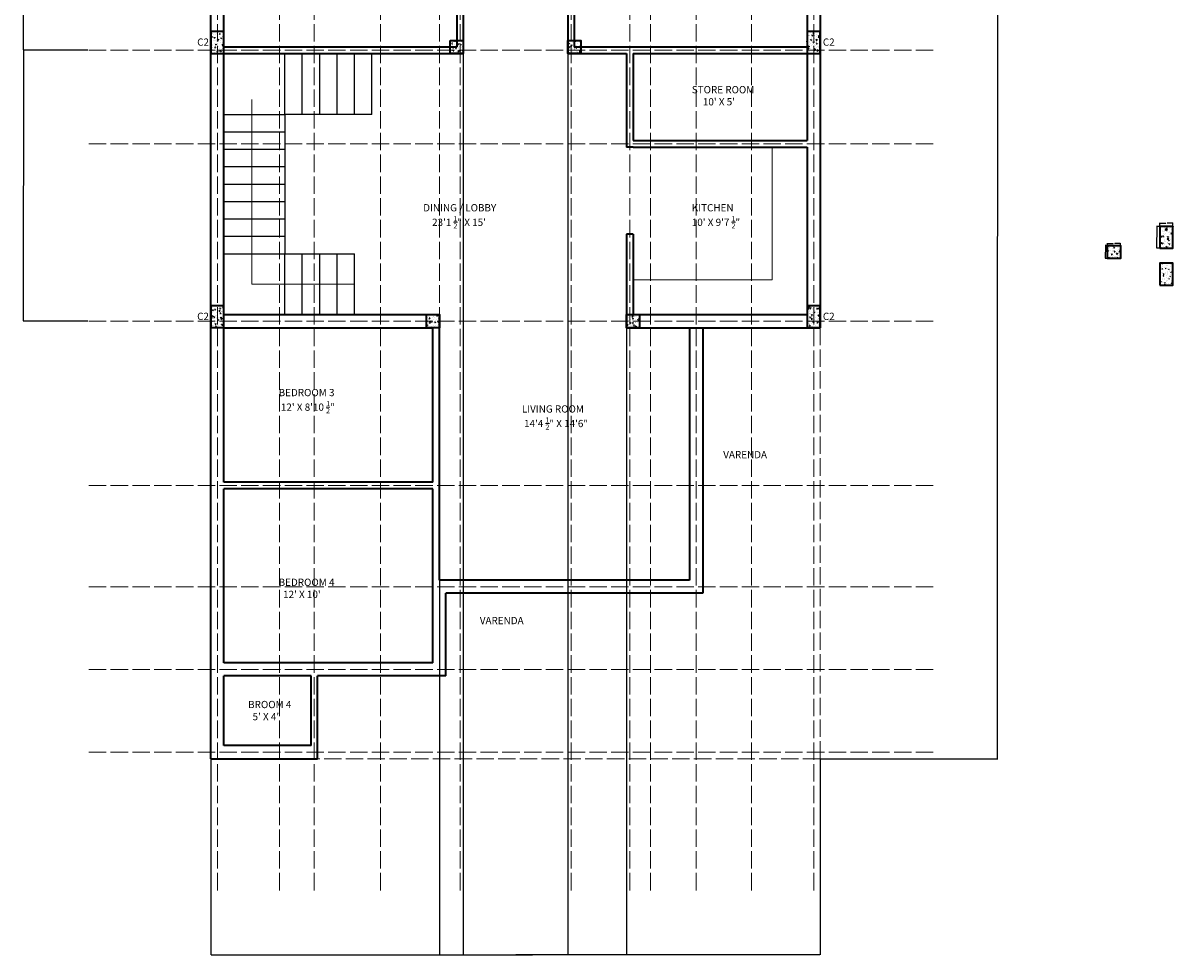
# Model space of a CAD drawing. Units: inches. Extents: x 1159 to 4240, y 1112 to 2085.
# Tile 11 of 13: x 2561 to 3354, y 1112 to 1755. Entities that reach past the tile are written whole.
import ezdxf

# ---------------------------------------------------------------- set-up
doc = ezdxf.new("R2010")
doc.units = ezdxf.units.IN
doc.linetypes.add('ACAD_ISO02W100', pattern=[15, 12, -3])
for name, color, linetype, lineweight in [('A-ANNO-DIMS', 2, 'Continuous', 18), ('A-ANNO-SYMB', 150, 'Continuous', 18), ('A-AREA-IDEN', 30, 'Continuous', 18), ('A-COLS-PATT', 120, 'Continuous', 13), ('A-FLOR-EDGE', 1, 'ACAD_ISO02W100', 18), ('A-GRID', 8, 'ACAD_ISO02W100', 13), ('COLUMN', 120, 'Continuous', 35), ('column no', 210, 'Continuous', 18), ('KITCHEN', 1, 'Continuous', 18), ('STAIRCASE', 150, 'Continuous', 25), ('WALL', 7, 'Continuous', 35)]:
    doc.layers.add(name, color=color, linetype=linetype, lineweight=lineweight)
doc.styles.get("Standard").update_dxf_attribs({"font": 'arial.ttf'})
doc.dimstyles.get("Standard").update_dxf_attribs({"dimtxt": 0.18, "dimasz": 0.18, "dimexe": 0.18, "dimexo": 0.0625, "dimgap": 0.09, "dimtad": 0, "dimtih": 1, "dimtoh": 1, "dimdec": 4, "dimzin": 0, "dimdsep": 46, "dimtxsty": 'Standard', "dimcen": 0.09, "dimadec": 0, "dimazin": 0, "dimtfac": 1, "dimtdec": 4, "dimtofl": 0, "dimtmove": 0, "dimatfit": 3, "dimfxl": 1, "dimtolj": 1, "dimtzin": 0, "dimarcsym": 0})

# ---------------------------------------------------------------- blocks, each defined once
blk = doc.blocks.new('column')
at = {"layer": 'COLUMN'}
h = blk.add_hatch(dxfattribs=at)
h.set_pattern_fill('AR-CONC', color=256, scale=0.025)
h.set_pattern_definition([(50, (-3308.5408, -1592.3894), (4.5546167, -0.398477), [0.47625, -5.23875]), (355, (-3308.541, -1592.3894), (-0.8810855, 4.776421), [0.381, -4.1910146]), (100.45144, (-3308.1612, -1592.4226), (3.673531, 4.377944), [0.40475, -4.452256]), (46.1842, (-3308.541, -1591.1194), (6.776976, -1.051058), [0.714375, -7.858125]), (96.63556, (-3307.976, -1591.207), (5.935103, 6.185653), [0.607126, -6.67839]), (351.18415, (-3308.541, -1591.1194), (5.935103, 6.185653), [0.571499, -6.286493]), (21, (-3307.9058, -1591.437), (3.7903598, -2.55663), [0.47625, -5.23875]), (326, (-3307.906, -1591.437), (1.545051, 4.604699), [0.381, -4.191]), (71.45144, (-3307.59, -1591.65), (5.3354105, 2.048069), [0.40475, -4.4522484]), (37.5, (-3308.5408, -1592.3894), (0.0772151, 2.113876), [0, -4.1402, 0, -4.2545, 0, -4.206875]), (7.5, (-3308.5408, -1592.3894), (1.6704916, 2.5045144), [0, -2.4257, 0, -4.04495, 0, -1.603375]), (327.5, (-3309.9568, -1592.3894), (3.3897649, -0.1432186), [0, -1.5875, 0, -4.953, 0, -6.57225]), (317.5, (-3310.5918, -1592.3894), (3.7032295, 0.6356623), [0, -2.06375, 0, -3.2893, 0, -4.66725])])
h.paths.add_polyline_path([(0, 9), (0, 0), (9, 0), (9, 9)])
blk.add_lwpolyline([(0, 9), (9, 9), (9, 0), (0, 0)], close=True, dxfattribs=at)
blk = doc.blocks.new('colum 1')
at = {"layer": 'COLUMN'}
h = blk.add_hatch(dxfattribs=at)
h.set_pattern_fill('AR-CONC', color=256, scale=0.025)
h.set_pattern_definition([(50, (-3344.692, -1599.4877), (4.5546167, -0.398477), [0.47625, -5.23875]), (355, (-3344.692, -1599.4877), (-0.8810855, 4.776421), [0.381, -4.1910146]), (100.45144, (-3344.3125, -1599.521), (3.673531, 4.377944), [0.40475, -4.452256]), (46.1842, (-3344.692, -1598.218), (6.776976, -1.051058), [0.714375, -7.858125]), (96.63556, (-3344.127, -1598.305), (5.935103, 6.185653), [0.607126, -6.67839]), (351.18415, (-3344.692, -1598.218), (5.935103, 6.185653), [0.571499, -6.286493]), (21, (-3344.057, -1598.5352), (3.7903598, -2.55663), [0.47625, -5.23875]), (326, (-3344.057, -1598.5352), (1.545051, 4.604699), [0.381, -4.191]), (71.45144, (-3343.741, -1598.7483), (5.3354105, 2.048069), [0.40475, -4.4522484]), (37.5, (-3344.692, -1599.4877), (0.0772151, 2.113876), [0, -4.1402, 0, -4.2545, 0, -4.206875]), (7.5, (-3344.692, -1599.4877), (1.6704916, 2.5045144), [0, -2.4257, 0, -4.04495, 0, -1.603375]), (327.5, (-3346.1081, -1599.4877), (3.3897649, -0.1432186), [0, -1.5875, 0, -4.953, 0, -6.57225]), (317.5, (-3346.743, -1599.4877), (3.7032295, 0.6356623), [0, -2.06375, 0, -3.2893, 0, -4.66725])])
h.paths.add_polyline_path([(9, 15), (0, 15), (0, 0), (9, 0)])
blk.add_lwpolyline([(0, 0), (9, 0), (9, 15), (0, 15)], close=True, dxfattribs=at)
blk = doc.blocks.new('HOUSE-35x60-WALL-LAYOUT')
for p, q in [((0, 0), (0, 720)), ((0, 720), (420, 720)), ((420, 720), (420, 297)), ((9, 711), (45, 711)), ((9, 634.5), (9, 711)), ((45, 634.5), (45, 711)), ((49.5, 639), (49.5, 711)), ((49.5, 711), (112.5, 711)), ((112.5, 639), (112.5, 711)), ((121.5, 639), (121.5, 711)), ((121.5, 711), (298.5, 711)), ((298.5, 711), (298.5, 639)), ((307.5, 711), (307.5, 639)), ((307.5, 711), (370.5, 711)), ((370.5, 711), (370.5, 639)), ((375, 711), (375, 634.5)), ((375, 711), (411, 711)), ((411, 711), (411, 634.5)), ((9, 490.5), (9, 634.5)), ((45, 634.5), (169.5, 634.5)), ((49.5, 639), (112.5, 639)), ((121.5, 639), (298.5, 639)), ((169.5, 634.5), (169.5, 490.5)), ((174, 634.5), (174, 531)), ((174, 634.5), (246, 634.5)), ((246, 634.5), (246, 531)), ((250.5, 634.5), (250.5, 490.5)), ((250.5, 634.5), (375, 634.5)), ((307.5, 639), (370.5, 639)), ((411, 634.5), (411, 490.5)), ((174, 531), (246, 531)), ((174, 526.5), (246, 526.5)), ((174, 526.5), (174, 486)), ((246, 526.5), (246, 486)), ((9, 490.5), (169.5, 490.5)), ((9, 486), (174, 486)), ((9, 306), (9, 486)), ((246, 486), (286.5, 486)), ((250.5, 490.5), (411, 490.5)), ((286.5, 486), (286.5, 421.5)), ((291, 486), (291, 426)), ((291, 486), (411, 486)), ((411, 486), (411, 426)), ((291, 421.5), (286.5, 421.5)), ((291, 426), (411, 426)), ((291, 421.5), (411, 421.5)), ((411, 421.5), (411, 306)), ((291, 361.5), (286.5, 361.5)), ((286.5, 361.5), (286.5, 297)), ((291, 361.5), (291, 306)), ((9, 306), (157.5, 306)), ((157.5, 190.5), (157.5, 306)), ((291, 306), (411, 306)), ((9, 297), (153, 297)), ((9, 190.5), (9, 297)), ((153, 190.5), (153, 297)), ((286.5, 297), (420, 297)), ((330, 297), (330, 123)), ((339, 297), (339, 114)), ((153, 190.5), (9, 190.5)), ((157.5, 123), (157.5, 190.5)), ((9, 66), (9, 186)), ((153, 186), (9, 186)), ((153, 66), (153, 186)), ((330, 123), (157.5, 123)), ((162, 57), (162, 114)), ((339, 114), (162, 114)), ((153, 66), (9, 66)), ((9, 9), (9, 57)), ((69, 57), (9, 57)), ((69, 9), (69, 57)), ((162, 57), (73.5, 57)), ((73.5, 0), (73.5, 57)), ((69, 9), (9, 9)), ((0, 0), (73.5, 0))]:
    blk.add_line(p, q)
blk = doc.blocks.new('STAIR-THREE-FLIGHT')
for p, q in [((42, 138), (42, 180)), ((54, 138), (54, 180)), ((66, 138), (66, 180)), ((78, 138), (78, 180)), ((90, 138), (90, 180)), ((102, 138), (102, 180)), ((0, 138), (42, 138)), ((102, 138), (42, 138)), ((42, 138), (42, 42)), ((0, 126), (42, 126)), ((0, 114), (42, 114)), ((0, 102), (42, 102)), ((0, 90), (42, 90)), ((0, 78), (42, 78)), ((0, 66), (42, 66)), ((0, 54), (42, 54)), ((0, 42), (42, 42)), ((42, 0), (42, 42)), ((42, 42), (90, 42)), ((54, 0), (54, 42)), ((66, 0), (66, 42)), ((78, 0), (78, 42)), ((90, 0), (90, 42))]:
    blk.add_line(p, q)
blk = doc.blocks.new('STAIR-PATH-ARROW')
blk.add_lwpolyline([(0, 127.38, 0, 0, 0), (0, 143.35, 0, 0, 0), (58.69, 143.35, 4, 0, 0), (70.69, 143.35, 0, 0, 0)], format="xyseb")
blk.add_lwpolyline([(70.69, 0), (0, 0), (0, 127.38)])
blk = doc.blocks.new('KITCHEN-COUNTER-L')
for p in [(96, 91.5), (0, 0)]:
    blk.add_line(p, (96, 0))
blk = doc.blocks.new('HOUSE-35x60-SETTING-OUT-GRID')
for p, q in [((89.32, 0), (89.32, 883.25)), ((132.07, 0), (132.07, 883.25)), ((156.07, 0), (156.07, 883.25)), ((201.82, 0), (201.82, 883.25)), ((242.32, 0), (242.32, 883.25)), ((256.57, 0), (256.57, 883.25)), ((333.07, 0), (333.07, 883.25)), ((373.57, 0), (373.57, 883.25)), ((387.82, 0), (387.82, 883.25)), ((419.32, 0), (419.32, 883.25)), ((457.57, 0), (457.57, 883.25)), ((500.32, 0), (500.32, 883.25)), ((582.7, 806.25), (0, 806.25)), ((582.7, 727.5), (0, 727.5)), ((582.7, 619.5), (0, 619.5)), ((582.7, 579), (0, 579)), ((582.7, 514.5), (0, 514.5)), ((582.7, 392.25), (0, 392.25)), ((582.7, 279), (0, 279)), ((582.7, 209.25), (0, 209.25)), ((582.7, 152.25), (0, 152.25)), ((582.7, 95.25), (0, 95.25))]:
    blk.add_line(p, q)
blk = doc.blocks.new('*D12')
at = {"layer": 'A-ANNO-DIMS', "color": 0, "lineweight": -2, "transparency": 16777216}
for p, q in [((3308.54, 1601.45), (3308.54, 1602.92)), ((3308.72, 1602.74), (3312.39, 1602.74)), ((3317.36, 1602.74), (3313.69, 1602.74)), ((3317.54, 1601.45), (3317.54, 1602.92))]:
    blk.add_line(p, q, dxfattribs=at)
at = {"layer": 'A-ANNO-DIMS', "color": 0, "lineweight": 100, "transparency": 16777216}
for points in [[(3308.72, 1602.77), (3308.72, 1602.71), (3308.54, 1602.74)], [(3317.36, 1602.77), (3317.36, 1602.71), (3317.54, 1602.74)]]:
    blk.add_solid(points, dxfattribs=at)
at = {"layer": 'Defpoints', "color": 0, "lineweight": 100, "transparency": 16777216}
for p in [(3308.54, 1601.39), (3317.54, 1602.74), (3317.54, 1601.39)]:
    blk.add_point(p, dxfattribs=at)
at = {"layer": 'A-ANNO-DIMS', "color": 0, "transparency": 16777216, "insert": (3313.04, 1602.74), "char_height": 0.18, "attachment_point": 5}
blk.add_mtext('\\A1;C1 9 TYP.', dxfattribs=at)
blk = doc.blocks.new('*D13')
at = {"layer": 'A-ANNO-DIMS', "color": 0, "lineweight": -2, "transparency": 16777216}
for p, q in [((3308.48, 1601.39), (3307.01, 1601.39)), ((3307.19, 1601.21), (3307.19, 1597.07)), ((3307.19, 1592.57), (3307.19, 1596.71)), ((3308.48, 1592.39), (3307.01, 1592.39))]:
    blk.add_line(p, q, dxfattribs=at)
at = {"layer": 'A-ANNO-DIMS', "color": 0, "lineweight": 100, "transparency": 16777216}
for points in [[(3307.16, 1601.21), (3307.22, 1601.21), (3307.19, 1601.39)], [(3307.16, 1592.57), (3307.22, 1592.57), (3307.19, 1592.39)]]:
    blk.add_solid(points, dxfattribs=at)
at = {"layer": 'Defpoints', "color": 0, "lineweight": 100, "transparency": 16777216}
for p in [(3307.19, 1601.39), (3308.54, 1601.39), (3308.54, 1592.39)]:
    blk.add_point(p, dxfattribs=at)
at = {"layer": 'A-ANNO-DIMS', "color": 0, "transparency": 16777216, "insert": (3307.19, 1596.89), "char_height": 0.18, "attachment_point": 5}
blk.add_mtext('\\A1;9 TYP.', dxfattribs=at)
blk = doc.blocks.new('*D14')
at = {"layer": 'A-ANNO-DIMS', "color": 0, "lineweight": -2, "transparency": 16777216}
for p, q in [((3344.63, 1614.49), (3342.26, 1614.49)), ((3342.44, 1614.31), (3342.44, 1607.17)), ((3342.44, 1599.67), (3342.44, 1606.8)), ((3344.63, 1599.49), (3342.26, 1599.49))]:
    blk.add_line(p, q, dxfattribs=at)
at = {"layer": 'A-ANNO-DIMS', "color": 0, "lineweight": 100, "transparency": 16777216}
for points in [[(3342.41, 1614.31), (3342.47, 1614.31), (3342.44, 1614.49)], [(3342.41, 1599.67), (3342.47, 1599.67), (3342.44, 1599.49)]]:
    blk.add_solid(points, dxfattribs=at)
at = {"layer": 'Defpoints', "color": 0, "lineweight": 100, "transparency": 16777216}
for p in [(3342.44, 1614.49), (3344.69, 1614.49), (3344.69, 1599.49)]:
    blk.add_point(p, dxfattribs=at)
at = {"layer": 'A-ANNO-DIMS', "color": 0, "transparency": 16777216, "insert": (3342.44, 1606.99), "char_height": 0.18, "attachment_point": 5}
blk.add_mtext('\\A1;C2 15 TYP.', dxfattribs=at)
blk = doc.blocks.new('*D15')
at = {"layer": 'A-ANNO-DIMS', "color": 0, "lineweight": -2, "transparency": 16777216}
for p, q in [((3344.69, 1614.55), (3344.69, 1616.92)), ((3344.87, 1616.74), (3348.73, 1616.74)), ((3353.51, 1616.74), (3349.65, 1616.74)), ((3353.69, 1614.55), (3353.69, 1616.92))]:
    blk.add_line(p, q, dxfattribs=at)
at = {"layer": 'A-ANNO-DIMS', "color": 0, "lineweight": 100, "transparency": 16777216}
for points in [[(3344.87, 1616.77), (3344.87, 1616.71), (3344.69, 1616.74)], [(3353.51, 1616.77), (3353.51, 1616.71), (3353.69, 1616.74)]]:
    blk.add_solid(points, dxfattribs=at)
at = {"layer": 'Defpoints', "color": 0, "lineweight": 100, "transparency": 16777216}
for p in [(3344.69, 1614.49), (3353.69, 1616.74), (3353.69, 1614.49)]:
    blk.add_point(p, dxfattribs=at)
at = {"layer": 'A-ANNO-DIMS', "color": 0, "transparency": 16777216, "insert": (3349.19, 1616.74), "char_height": 0.18, "attachment_point": 5}
blk.add_mtext('\\A1;9 TYP.', dxfattribs=at)
blk = doc.blocks.new('*D24')
at = {"layer": 'A-ANNO-DIMS', "color": 0, "lineweight": -2, "transparency": 16777216}
for p, q in [((2690.48, 1247.64), (2690.48, 1112.42)), ((3110.48, 1247.64), (3110.48, 1112.42)), ((2690.66, 1112.6), (2900.19, 1112.6)), ((3110.3, 1112.6), (2900.78, 1112.6))]:
    blk.add_line(p, q, dxfattribs=at)
at = {"layer": 'A-ANNO-DIMS', "color": 0, "lineweight": 100, "transparency": 16777216}
for points in [[(2690.66, 1112.63), (2690.66, 1112.57), (2690.48, 1112.6)], [(3110.3, 1112.63), (3110.3, 1112.57), (3110.48, 1112.6)]]:
    blk.add_solid(points, dxfattribs=at)
at = {"layer": 'Defpoints', "color": 0, "lineweight": 100, "transparency": 16777216}
for p in [(2690.48, 1247.7), (3110.48, 1247.7), (3110.48, 1112.6)]:
    blk.add_point(p, dxfattribs=at)
at = {"layer": 'A-ANNO-DIMS', "color": 0, "transparency": 16777216, "insert": (2900.48, 1112.6), "char_height": 0.18, "attachment_point": 5}
blk.add_mtext('\\A1;420', dxfattribs=at)
blk = doc.blocks.new('*D25')
at = {"layer": 'A-ANNO-DIMS', "color": 0, "lineweight": -2, "transparency": 16777216}
for p, q in [((3110.55, 1967.7), (3232.9, 1967.7)), ((3232.72, 1967.52), (3232.72, 1607.88)), ((3232.72, 1247.88), (3232.72, 1607.52)), ((3110.55, 1247.7), (3232.9, 1247.7))]:
    blk.add_line(p, q, dxfattribs=at)
at = {"layer": 'A-ANNO-DIMS', "color": 0, "lineweight": 100, "transparency": 16777216}
for points in [[(3232.69, 1967.52), (3232.75, 1967.52), (3232.72, 1967.7)], [(3232.69, 1247.88), (3232.75, 1247.88), (3232.72, 1247.7)]]:
    blk.add_solid(points, dxfattribs=at)
at = {"layer": 'Defpoints', "color": 0, "lineweight": 100, "transparency": 16777216}
for p in [(3110.48, 1967.7), (3232.72, 1967.7), (3110.48, 1247.7)]:
    blk.add_point(p, dxfattribs=at)
at = {"layer": 'A-ANNO-DIMS', "color": 0, "transparency": 16777216, "insert": (3232.72, 1607.7), "char_height": 0.18, "attachment_point": 5}
blk.add_mtext('\\A1;720', dxfattribs=at)
blk = doc.blocks.new('*D49')
at = {"layer": 'A-ANNO-DIMS', "color": 0, "lineweight": -2, "transparency": 16777216}
for p, q in [((2605.61, 1735.95), (2561.14, 1735.95)), ((2561.32, 1735.77), (2561.32, 1642.76)), ((2561.32, 1549.38), (2561.32, 1642.4)), ((2605.61, 1549.2), (2561.14, 1549.2))]:
    blk.add_line(p, q, dxfattribs=at)
at = {"layer": 'A-ANNO-DIMS', "color": 0, "lineweight": 100, "transparency": 16777216}
for points in [[(2561.29, 1735.77), (2561.35, 1735.77), (2561.32, 1735.95)], [(2561.29, 1549.38), (2561.35, 1549.38), (2561.32, 1549.2)]]:
    blk.add_solid(points, dxfattribs=at)
at = {"layer": 'Defpoints', "color": 0, "lineweight": 100, "transparency": 16777216}
for p in [(2561.32, 1735.95), (2605.67, 1735.95), (2605.67, 1549.2)]:
    blk.add_point(p, dxfattribs=at)
at = {"layer": 'A-ANNO-DIMS', "color": 0, "transparency": 16777216, "insert": (2561.32, 1642.58), "char_height": 0.18, "attachment_point": 5}
blk.add_mtext('\\A1;186.75', dxfattribs=at)
blk = doc.blocks.new('*D50')
at = {"layer": 'A-ANNO-DIMS', "color": 0, "lineweight": -2, "transparency": 16777216}
for p, q in [((2605.61, 1884.45), (2561.14, 1884.45)), ((2561.32, 1884.27), (2561.32, 1810.38)), ((2561.32, 1736.13), (2561.32, 1810.02)), ((2605.61, 1735.95), (2561.14, 1735.95))]:
    blk.add_line(p, q, dxfattribs=at)
at = {"layer": 'A-ANNO-DIMS', "color": 0, "lineweight": 100, "transparency": 16777216}
for points in [[(2561.29, 1884.27), (2561.35, 1884.27), (2561.32, 1884.45)], [(2561.29, 1736.13), (2561.35, 1736.13), (2561.32, 1735.95)]]:
    blk.add_solid(points, dxfattribs=at)
at = {"layer": 'Defpoints', "color": 0, "lineweight": 100, "transparency": 16777216}
for p in [(2561.32, 1884.45), (2605.67, 1884.45), (2605.67, 1735.95)]:
    blk.add_point(p, dxfattribs=at)
at = {"layer": 'A-ANNO-DIMS', "color": 0, "transparency": 16777216, "insert": (2561.32, 1810.2), "char_height": 0.18, "attachment_point": 5}
blk.add_mtext('\\A1;148.5', dxfattribs=at)
blk = doc.blocks.new('*D53')
at = {"layer": 'A-ANNO-DIMS', "color": 0, "lineweight": -2, "transparency": 16777216}
for p, q in [((2864.48, 1733.64), (2864.48, 1112.42)), ((2936.48, 1733.64), (2936.48, 1112.42)), ((2864.66, 1112.6), (2900.27, 1112.6)), ((2936.3, 1112.6), (2900.7, 1112.6))]:
    blk.add_line(p, q, dxfattribs=at)
at = {"layer": 'A-ANNO-DIMS', "color": 0, "lineweight": 100, "transparency": 16777216}
for points in [[(2864.66, 1112.63), (2864.66, 1112.57), (2864.48, 1112.6)], [(2936.3, 1112.63), (2936.3, 1112.57), (2936.48, 1112.6)]]:
    blk.add_solid(points, dxfattribs=at)
at = {"layer": 'Defpoints', "color": 0, "lineweight": 100, "transparency": 16777216}
for p in [(2864.48, 1733.7), (2936.48, 1733.7), (2936.48, 1112.6)]:
    blk.add_point(p, dxfattribs=at)
at = {"layer": 'A-ANNO-DIMS', "color": 0, "transparency": 16777216, "insert": (2900.48, 1112.6), "char_height": 0.18, "attachment_point": 5}
blk.add_mtext('\\A1;72', dxfattribs=at)
blk = doc.blocks.new('*D54')
at = {"layer": 'A-ANNO-DIMS', "color": 0, "lineweight": -2, "transparency": 16777216}
for p, q in [((2847.98, 1544.64), (2847.98, 1112.42)), ((2976.98, 1544.64), (2976.98, 1112.42)), ((2848.16, 1112.6), (2912.2, 1112.6)), ((2976.8, 1112.6), (2912.76, 1112.6))]:
    blk.add_line(p, q, dxfattribs=at)
at = {"layer": 'A-ANNO-DIMS', "color": 0, "lineweight": 100, "transparency": 16777216}
for points in [[(2848.16, 1112.63), (2848.16, 1112.57), (2847.98, 1112.6)], [(2976.8, 1112.63), (2976.8, 1112.57), (2976.98, 1112.6)]]:
    blk.add_solid(points, dxfattribs=at)
at = {"layer": 'Defpoints', "color": 0, "lineweight": 100, "transparency": 16777216}
for p in [(2847.98, 1544.7), (2976.98, 1544.7), (2976.98, 1112.6)]:
    blk.add_point(p, dxfattribs=at)
at = {"layer": 'A-ANNO-DIMS', "color": 0, "transparency": 16777216, "insert": (2912.48, 1112.6), "char_height": 0.18, "attachment_point": 5}
blk.add_mtext('\\A1;129', dxfattribs=at)

msp = doc.modelspace()

# ---------------------------------------------------------------- hatches: boundary and pattern name
at = {"layer": 'A-COLS-PATT'}
h = msp.add_hatch(dxfattribs=at)
h.set_pattern_fill('AR-CONC', color=256, scale=0.025)
h.set_pattern_definition([(50, (0, -25.3897), (4.5546167, -0.398477), [0.47625, -5.23875]), (355, (0, -25.3897), (-0.8810855, 4.776421), [0.381, -4.1910146]), (100.45144, (0.3796, -25.423), (3.673531, 4.377944), [0.40475, -4.452256]), (46.1842, (0, -24.1197), (6.776976, -1.051058), [0.714375, -7.858125]), (96.63556, (0.565, -24.207), (5.935103, 6.185653), [0.607126, -6.67839]), (351.18415, (0, -24.12), (5.935103, 6.185653), [0.571499, -6.286493]), (21, (0.635, -24.437), (3.7903598, -2.55663), [0.47625, -5.23875]), (326, (0.635, -24.437), (1.545051, 4.604699), [0.381, -4.191]), (71.45144, (0.951, -24.6502), (5.3354105, 2.048069), [0.40475, -4.4522484]), (37.5, (0, -25.3897), (0.0772151, 2.113876), [0, -4.1402, 0, -4.2545, 0, -4.206875]), (7.5, (0, -25.3897), (1.6704916, 2.5045144), [0, -2.4257, 0, -4.04495, 0, -1.603375]), (327.5, (-1.416, -25.3897), (3.3897649, -0.1432186), [0, -1.5875, 0, -4.953, 0, -6.57225]), (317.5, (-2.051, -25.3897), (3.7032295, 0.6356623), [0, -2.06375, 0, -3.2893, 0, -4.66725])])
h.paths.add_polyline_path([(3353.692, 1589.098), (3344.692, 1589.098), (3344.692, 1574.098), (3353.692, 1574.098)])

# ---------------------------------------------------------------- linework, layer by layer
at = {"layer": 'A-FLOR-EDGE'}
for p, q in [((3110.484, 1544.702), (3110.484, 1247.702)), ((3110.484, 1247.702), (2763.984, 1247.702))]:
    msp.add_line(p, q, dxfattribs=at)
at = {"layer": 'COLUMN'}
msp.add_lwpolyline([(3344.692, 1574.098), (3353.692, 1574.098), (3353.692, 1589.098), (3344.692, 1589.098)], close=True, dxfattribs=at)

# ---------------------------------------------------------------- block references
at = {"layer": 'A-ANNO-SYMB'}
msp.add_blockref('STAIR-PATH-ARROW', (2718.795, 1574.702), dxfattribs=at)
at = {"layer": 'A-GRID'}
msp.add_blockref('HOUSE-35x60-SETTING-OUT-GRID', (2605.668, 1156.954), dxfattribs=at)
at = {"layer": 'COLUMN'}
for name, p in [('colum 1', (2690.484, 1733.733)), ('colum 1', (3101.484, 1733.733)), ('column', (2855.484, 1733.702)), ('column', (2936.484, 1733.702)), ('colum 1', (3344.692, 1599.488)), ('column', (3308.541, 1592.389)), ('colum 1', (2690.484, 1544.733)), ('colum 1', (3101.484, 1544.733)), ('column', (2838.984, 1544.702)), ('column', (2976.984, 1544.702))]:
    msp.add_blockref(name, p, dxfattribs=at)
at = {"layer": 'KITCHEN'}
msp.add_blockref('KITCHEN-COUNTER-L', (2981.484, 1577.702), dxfattribs=at)
at = {"layer": 'STAIRCASE'}
msp.add_blockref('STAIR-THREE-FLIGHT', (2699.484, 1553.702), dxfattribs=at)
at = {"layer": 'WALL'}
msp.add_blockref('HOUSE-35x60-WALL-LAYOUT', (2690.484, 1247.702), dxfattribs=at)

# ---------------------------------------------------------------- texts
at = {"layer": 'A-AREA-IDEN', "char_height": 5, "attachment_point": 1}
for s, insert in [("\\A1;STORE ROOM\\P     10' X 5'", (3021.978, 1711.241)), ('\\A1;DINING / LOBBY\\P    23\'1 {\\H0.7x;\\S1/2;}" X 15\'', (2836.829, 1629.873)), ('\\A1;KITCHEN\\P10\' X 9\'7 {\\H0.7x;\\S1/2;}"', (3021.978, 1629.873)), ('\\A1;BEDROOM 3\\P 12\' X 8\'10 {\\H0.7x;\\S1/2;}"', (2737.175, 1502.503)), ('\\A1;LIVING ROOM\\P 14\'4 {\\H0.7x;\\S1/2;}" X 14\'6"', (2904.82, 1491.215)), ('\\A1;VARENDA', (3043.648, 1459.712)), ("\\A1;BEDROOM 4\\P  12' X 10'", (2737.175, 1371.76)), ('\\A1;VARENDA', (2875.841, 1345.387)), ("\\A1;BROOM 4 \\P  5' X 4'", (2716.13, 1287.528))]:
    msp.add_mtext_dynamic_manual_height_columns(s, width=140.18614, gutter_width=12.5, heights=[0], dxfattribs=dict(at, insert=insert))
at = {"layer": 'column no', "char_height": 5, "attachment_point": 1}
for insert in [(2681.009, 1744.032), (3112.322, 1744.032), (2681.009, 1555.032), (3112.322, 1555.032)]:
    msp.add_mtext_dynamic_manual_height_columns('\\A1;C2', width=140.18614, gutter_width=12.5, heights=[0], dxfattribs=dict(at, insert=insert))

# ---------------------------------------------------------------- dimensions: what is measured, and where the dimension line sits
at = {"layer": 'A-ANNO-DIMS'}
for base, p1, p2, override, picture, middle in [((3232.722, 1967.702), (3110.484, 1247.702), (3110.484, 1967.702), {"dimdec": 0, "dimlfac": 1, "dimrnd": 0, "dimzin": 0, "dimdsep": 46, "dimlunit": 2}, '*D25', (3232.722, 1607.702)), ((2561.318, 1884.452), (2605.668, 1735.952), (2605.668, 1884.452), {"dimdec": 1, "dimlfac": 1, "dimrnd": 0, "dimzin": 0, "dimdsep": 46, "dimlunit": 2}, '*D50', (2561.318, 1810.202)), ((2561.318, 1735.952), (2605.668, 1549.202), (2605.668, 1735.952), {"dimdec": 2, "dimlfac": 1, "dimrnd": 0, "dimzin": 0, "dimdsep": 46, "dimlunit": 2}, '*D49', (2561.318, 1642.577))]:
    dim = msp.add_linear_dim(base=base, p1=p1, p2=p2, angle=90, dimstyle='Standard', override=override, dxfattribs=at)
    dim.commit()
    dim.dimension.update_dxf_attribs({"geometry": picture, "text_midpoint": middle})
for base, p1, p2, picture, middle in [((2936.484, 1112.604), (2864.484, 1733.702), (2936.484, 1733.702), '*D53', (2900.484, 1112.604)), ((2976.984, 1112.604), (2847.984, 1544.702), (2976.984, 1544.702), '*D54', (2912.484, 1112.604)), ((3110.484, 1112.604), (2690.484, 1247.702), (3110.484, 1247.702), '*D24', (2900.484, 1112.604))]:
    dim = msp.add_linear_dim(base=base, p1=p1, p2=p2, dimstyle='Standard', override={"dimdec": 0, "dimlfac": 1, "dimrnd": 0, "dimzin": 0, "dimdsep": 46, "dimlunit": 2}, dxfattribs=at)
    dim.commit()
    dim.dimension.update_dxf_attribs({"geometry": picture, "text_midpoint": middle})
for base, p1, p2, text, picture, middle in [((3342.442, 1614.488), (3344.692, 1599.488), (3344.692, 1614.488), 'C2 <> TYP.', '*D14', (3342.442, 1606.988)), ((3307.191, 1601.389), (3308.541, 1592.389), (3308.541, 1601.389), '<> TYP.', '*D13', (3307.191, 1596.889))]:
    dim = msp.add_linear_dim(base=base, p1=p1, p2=p2, angle=90, text=text, dimstyle='Standard', override={"dimdec": 0, "dimlfac": 1, "dimrnd": 0, "dimzin": 0, "dimdsep": 46, "dimlunit": 2}, dxfattribs=at)
    dim.commit()
    dim.dimension.update_dxf_attribs({"geometry": picture, "text_midpoint": middle})
for base, p1, p2, text, picture, middle in [((3353.692, 1616.738), (3344.692, 1614.488), (3353.692, 1614.488), '<> TYP.', '*D15', (3349.192, 1616.738)), ((3317.541, 1602.739), (3308.541, 1601.389), (3317.541, 1601.389), 'C1 <> TYP.', '*D12', (3313.041, 1602.739))]:
    dim = msp.add_linear_dim(base=base, p1=p1, p2=p2, text=text, dimstyle='Standard', override={"dimdec": 0, "dimlfac": 1, "dimrnd": 0, "dimzin": 0, "dimdsep": 46, "dimlunit": 2}, dxfattribs=at)
    dim.commit()
    dim.dimension.update_dxf_attribs({"geometry": picture, "text_midpoint": middle})

doc.saveas('drawing.dxf')
